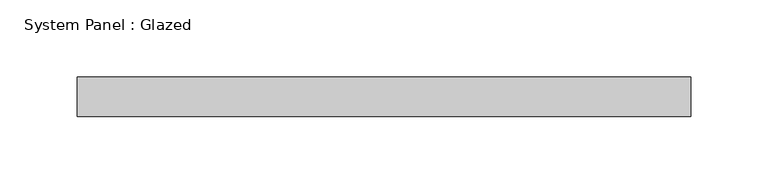
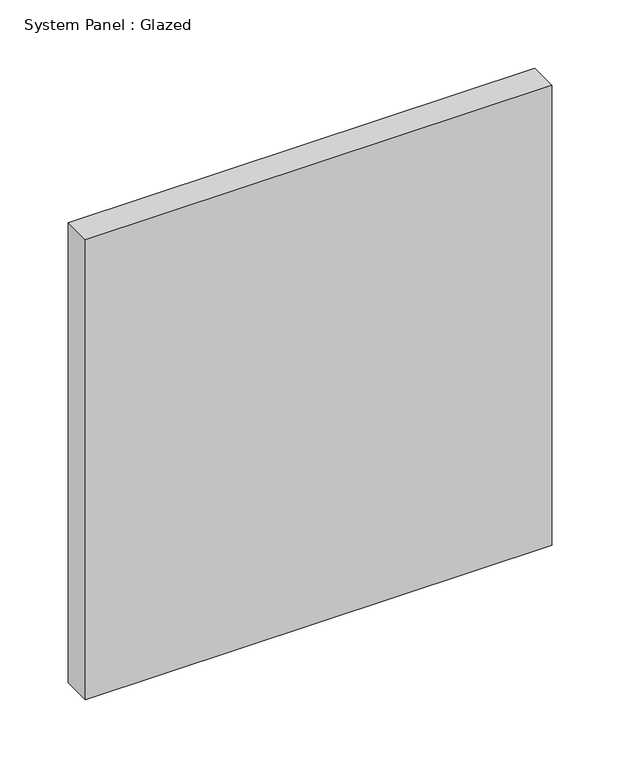
"""IFC4 building model written with IfcOpenShell, lengths in millimetres: plate geometry, System Panel : Glazed."""

from ifc_helpers import new_model, si_unit, origin, origin_with_axes, place, context, project, spatial, polyline, outline, extrude, source, transform, mapped, element, save


def system_panel_glazed_4258910c(model_context):
    return source(origin(), model_context, "Body", "SweptSolid", [
        extrude(outline(polyline([(197.9083333, 19.05), (-197.9083333, 19.05), (-197.9083333, 44.45), (197.9083333, 44.45), (197.9083333, 19.05)])), origin_with_axes(), (0.0, 0.0, 1.0), 412.75),
    ])


if __name__ == "__main__":
    model = new_model("IFC4")
    model_context = context("Model", 3, world=origin())
    ifc_project = project(units=[si_unit("LENGTHUNIT", "METRE", prefix="MILLI")], contexts=[model_context])
    site = spatial("IfcSite", under=ifc_project)
    building = spatial("IfcBuilding", under=site)
    placement = place(None, origin())
    system_panel_glazed_shape = system_panel_glazed_4258910c(model_context)
    element("IfcPlate", 1, ObjectType="System Panel : Glazed", at=placement, inside=building, context=model_context, shape_type="MappedRepresentation", body=[
        mapped(system_panel_glazed_shape, transform((0.0, 0.0, 0.0), x_axis=(1.0, 0.0, 0.0), y_axis=(0.0, 1.0, 0.0), z_axis=(0.0, 0.0, 1.0))),
    ])
    save(model, "model.ifc")

# Revit data of these elements
# Type "System Panel : Glazed"
#   Construction Type Id = "GSP4R"
#   Analytic Construction = "1/8 in Pilkington single glazing"
#   Visual Light Transmittance = 0.9
#   Solar Heat Gain Coefficient = 0.86
#   Heat Transfer Coefficient (U) = 1.18115 BTU/(h·ft²·°F)
#   Define Thermal Properties by = 1
# Element 1 (IfcPlate, "System Panel : Glazed")
#   Materials on its faces: "Glass"
# Materials
#   "Glass": class "Glass", colour RGB 0 128 192, transparency 0.75, Description = "Soda Lime Glass", Cost = 0
